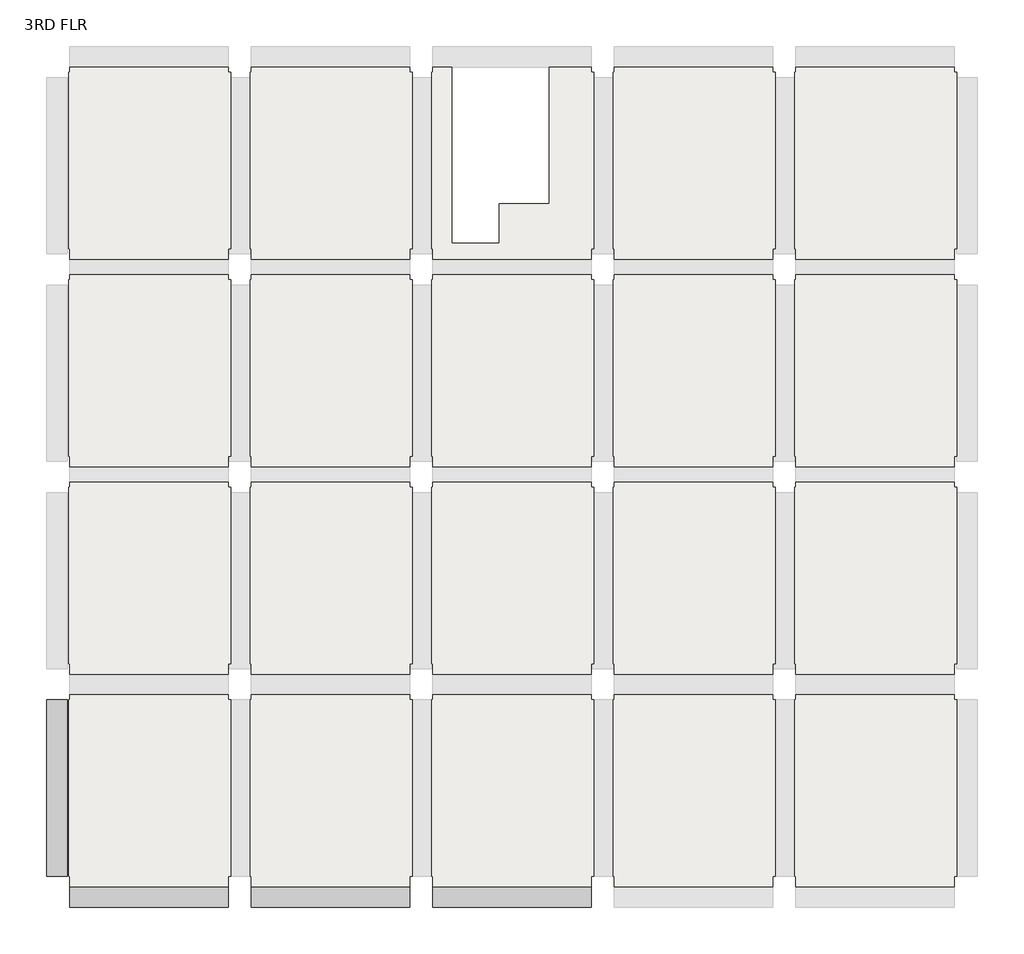
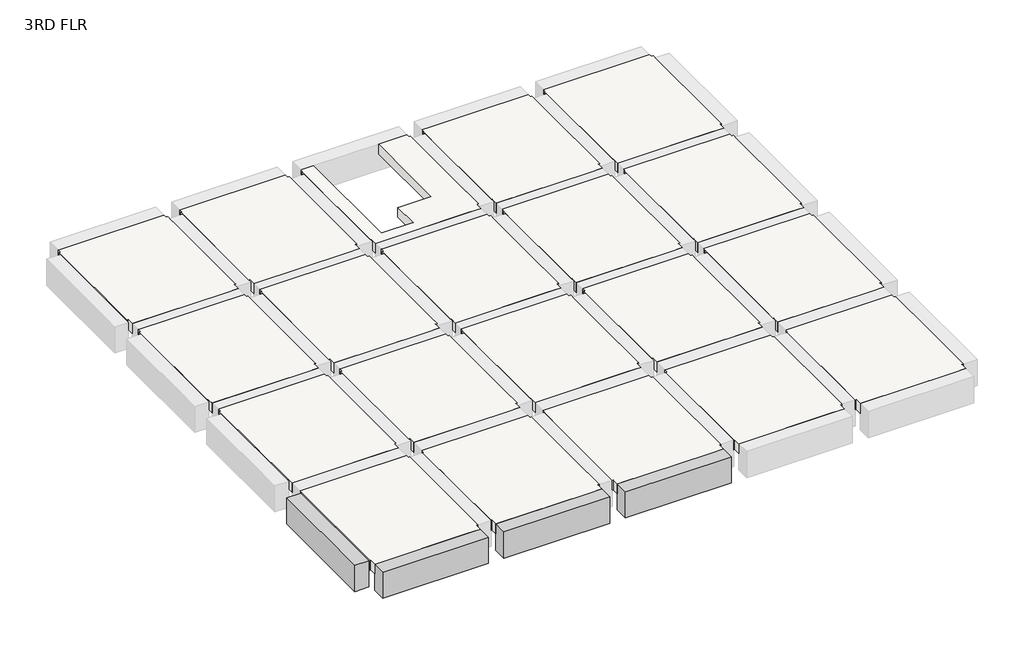
# One storey, part 1 of 2: 20 slabs, 4 beams.
"""IFC4 building model written with IfcOpenShell, lengths in millimetres."""

from ifc_helpers import new_model, si_unit, frame, origin, place, context, project, spatial, polyline, outline, extrude, faceted_brep, element, save

model = new_model("IFC4")

# Units and contexts
model_context = context("Model", 3, world=origin())
ifc_project = project(units=[si_unit("LENGTHUNIT", "METRE", prefix="MILLI")], contexts=[model_context])

# Site, building, storey
site = spatial("IfcSite", under=ifc_project)
building = spatial("IfcBuilding", under=site)
storey = spatial("IfcBuildingStorey", under=building, Name="3RD FLR", Elevation=9144.0)

# Beams
placement = place(None, origin())
element("IfcBeam", 1, ObjectType="M_Concrete-Rectangular Beam : 400 x 800mm", at=placement, inside=storey, context=model_context, shape_type="Brep", body=[
    faceted_brep([(-2144.8884094, 3503.1212443, 9144.0), (-2144.8884094, 3103.1212443, 9144.0), (905.1115906, 3103.1212443, 9144.0), (905.1115906, 3503.1212443, 9144.0), (-2144.8884094, 3503.1212443, 8344.0), (-2144.8884094, 3503.1212443, 8844.0), (905.1115906, 3503.1212443, 8844.0), (905.1115906, 3503.1212443, 8344.0), (-2144.8884094, 3103.1212443, 8344.0), (905.1115906, 3103.1212443, 8344.0)], [[[0, 1, 2, 3]], [[4, 5, 0, 3, 6, 7]], [[8, 4, 7, 9]], [[1, 8, 9, 2]], [[1, 0, 5, 4, 8]], [[3, 2, 9, 7, 6]]]),
])
element("IfcBeam", 2, ObjectType="M_Concrete-Rectangular Beam : 400 x 800mm", at=placement, inside=storey, context=model_context, shape_type="Brep", body=[
    faceted_brep([(-5644.8884094, 3503.1212443, 9144.0), (-5644.8884094, 3103.1212443, 9144.0), (-2594.8884094, 3103.1212443, 9144.0), (-2594.8884094, 3503.1212443, 9144.0), (-5644.8884094, 3503.1212443, 8344.0), (-5644.8884094, 3503.1212443, 8844.0), (-2594.8884094, 3503.1212443, 8844.0), (-2594.8884094, 3503.1212443, 8344.0), (-5644.8884094, 3103.1212443, 8344.0), (-2594.8884094, 3103.1212443, 8344.0)], [[[0, 1, 2, 3]], [[4, 5, 0, 3, 6, 7]], [[8, 4, 7, 9]], [[1, 8, 9, 2]], [[1, 0, 5, 4, 8]], [[3, 2, 9, 7, 6]]]),
])
element("IfcBeam", 3, ObjectType="M_Concrete-Rectangular Beam : 400 x 800mm", at=placement, inside=storey, context=model_context, shape_type="Brep", body=[
    faceted_brep([(-9144.8884094, 3503.1212443, 9144.0), (-9144.8884094, 3103.1212443, 9144.0), (-6094.8884094, 3103.1212443, 9144.0), (-6094.8884094, 3503.1212443, 9144.0), (-9144.8884094, 3503.1212443, 8344.0), (-9144.8884094, 3503.1212443, 8844.0), (-6094.8884094, 3503.1212443, 8844.0), (-6094.8884094, 3503.1212443, 8344.0), (-9144.8884094, 3103.1212443, 8344.0), (-6094.8884094, 3103.1212443, 8344.0)], [[[0, 1, 2, 3]], [[4, 5, 0, 3, 6, 7]], [[8, 4, 7, 9]], [[1, 8, 9, 2]], [[1, 0, 5, 4, 8]], [[3, 2, 9, 7, 6]]]),
])
element("IfcBeam", 4, ObjectType="M_Concrete-Rectangular Beam : 400 x 800mm", at=placement, inside=storey, context=model_context, shape_type="SweptSolid", body=[
    extrude(outline(polyline([(-9594.8884094, 7103.1212443), (-9194.8884094, 7103.1212443), (-9194.8884094, 3703.1212443), (-9594.8884094, 3703.1212443), (-9594.8884094, 7103.1212443)])), frame((0.0, 0.0, 8344.0), z_axis=(0.0, 0.0, 1.0), x_axis=(1.0, 0.0, 0.0)), (0.0, 0.0, 1.0), 800.0),
])

# Slabs
element("IfcSlab", 5, ObjectType="Generic 300mm", at=placement, inside=storey, context=model_context, shape_type="SweptSolid", body=[
    extrude(outline(polyline([(7955.1115906, 7103.1212443), (7955.1115906, 3703.1212443), (7905.1115906, 3703.1212443), (7905.1115906, 3503.1212443), (7530.1115906, 3503.1212443), (4855.1115906, 3503.1212443), (4855.1115906, 3703.1212443), (4830.1115906, 3703.1212443), (4830.1115906, 7103.1212443), (4855.1115906, 7103.1212443), (4855.1115906, 7203.1212443), (7905.1115906, 7203.1212443), (7905.1115906, 7103.1212443), (7955.1115906, 7103.1212443)])), frame((0.0, 0.0, 8844.0), z_axis=(0.0, 0.0, 1.0), x_axis=(1.0, 0.0, 0.0)), (0.0, 0.0, 1.0), 300.0),
])
element("IfcSlab", 6, ObjectType="Generic 300mm", at=placement, inside=storey, context=model_context, shape_type="Brep", body=[
    faceted_brep([(7955.1115906, 11203.1212443, 8844.0), (7955.1115906, 11103.1212443, 8844.0), (7955.1115906, 7803.1212443, 8844.0), (7905.1115906, 7803.1212443, 8844.0), (7905.1115906, 7603.1212443, 8844.0), (7530.1115906, 7603.1212443, 8844.0), (4855.1115906, 7603.1212443, 8844.0), (4855.1115906, 7803.1212443, 8844.0), (4830.1115906, 7803.1212443, 8844.0), (4830.1115906, 11103.1212443, 8844.0), (4830.1115906, 11203.1212443, 8844.0), (4855.1115906, 11203.1212443, 8844.0), (4855.1115906, 11303.1212443, 8844.0), (7905.1115906, 11303.1212443, 8844.0), (7905.1115906, 11203.1212443, 8844.0), (7955.1115906, 11203.1212443, 9144.0), (7905.1115906, 11203.1212443, 9144.0), (7905.1115906, 11303.1212443, 9144.0), (4855.1115906, 11303.1212443, 9144.0), (4855.1115906, 11203.1212443, 9144.0), (4830.1115906, 11203.1212443, 9144.0), (4830.1115906, 11103.1212443, 9144.0), (4830.1115906, 7803.1212443, 9144.0), (4855.1115906, 7803.1212443, 9144.0), (4855.1115906, 7703.1212443, 9144.0), (4855.1115906, 7603.1212443, 9144.0), (7530.1115906, 7603.1212443, 9144.0), (7905.1115906, 7603.1212443, 9144.0), (7905.1115906, 7703.1212443, 9144.0), (7905.1115906, 7803.1212443, 9144.0), (7955.1115906, 7803.1212443, 9144.0), (7955.1115906, 11103.1212443, 9144.0)], [[[0, 1, 2, 3, 4, 5, 6, 7, 8, 9, 10, 11, 12, 13, 14]], [[15, 16, 17, 18, 19, 20, 21, 22, 23, 24, 25, 26, 27, 28, 29, 30, 31]], [[2, 1, 0, 15, 31, 30]], [[3, 2, 30, 29]], [[4, 3, 29, 28, 27]], [[5, 4, 27, 26]], [[6, 5, 26, 25]], [[7, 6, 25, 24, 23]], [[8, 7, 23, 22]], [[10, 9, 8, 22, 21, 20]], [[11, 10, 20, 19]], [[12, 11, 19, 18]], [[13, 12, 18, 17]], [[14, 13, 17, 16]], [[0, 14, 16, 15]]]),
])
element("IfcSlab", 7, ObjectType="Generic 300mm", at=placement, inside=storey, context=model_context, shape_type="Brep", body=[
    faceted_brep([(4455.1115906, 11203.1212443, 8844.0), (4455.1115906, 11103.1212443, 8844.0), (4455.1115906, 7803.1212443, 8844.0), (4430.1115906, 7803.1212443, 8844.0), (4405.1115906, 7803.1212443, 8844.0), (4405.1115906, 7603.1212443, 8844.0), (4030.1115906, 7603.1212443, 8844.0), (1355.1115906, 7603.1212443, 8844.0), (1355.1115906, 7803.1212443, 8844.0), (1330.1115906, 7803.1212443, 8844.0), (1330.1115906, 11103.1212443, 8844.0), (1330.1115906, 11203.1212443, 8844.0), (1355.1115906, 11203.1212443, 8844.0), (1355.1115906, 11303.1212443, 8844.0), (4405.1115906, 11303.1212443, 8844.0), (4405.1115906, 11203.1212443, 8844.0), (4455.1115906, 11203.1212443, 9144.0), (4405.1115906, 11203.1212443, 9144.0), (4405.1115906, 11303.1212443, 9144.0), (1355.1115906, 11303.1212443, 9144.0), (1355.1115906, 11203.1212443, 9144.0), (1330.1115906, 11203.1212443, 9144.0), (1330.1115906, 11103.1212443, 9144.0), (1330.1115906, 7803.1212443, 9144.0), (1355.1115906, 7803.1212443, 9144.0), (1355.1115906, 7703.1212443, 9144.0), (1355.1115906, 7603.1212443, 9144.0), (4030.1115906, 7603.1212443, 9144.0), (4405.1115906, 7603.1212443, 9144.0), (4405.1115906, 7703.1212443, 9144.0), (4405.1115906, 7803.1212443, 9144.0), (4430.1115906, 7803.1212443, 9144.0), (4455.1115906, 7803.1212443, 9144.0), (4455.1115906, 11103.1212443, 9144.0)], [[[0, 1, 2, 3, 4, 5, 6, 7, 8, 9, 10, 11, 12, 13, 14, 15]], [[16, 17, 18, 19, 20, 21, 22, 23, 24, 25, 26, 27, 28, 29, 30, 31, 32, 33]], [[2, 1, 0, 16, 33, 32]], [[4, 3, 2, 32, 31, 30]], [[5, 4, 30, 29, 28]], [[6, 5, 28, 27]], [[7, 6, 27, 26]], [[8, 7, 26, 25, 24]], [[9, 8, 24, 23]], [[11, 10, 9, 23, 22, 21]], [[12, 11, 21, 20]], [[13, 12, 20, 19]], [[14, 13, 19, 18]], [[15, 14, 18, 17]], [[0, 15, 17, 16]]]),
])
element("IfcSlab", 8, ObjectType="Generic 300mm", at=placement, inside=storey, context=model_context, shape_type="Brep", body=[
    faceted_brep([(955.1115906, 11203.1212443, 8844.0), (955.1115906, 11103.1212443, 8844.0), (955.1115906, 7803.1212443, 8844.0), (930.1115906, 7803.1212443, 8844.0), (905.1115906, 7803.1212443, 8844.0), (905.1115906, 7603.1212443, 8844.0), (530.1115906, 7603.1212443, 8844.0), (-2144.8884094, 7603.1212443, 8844.0), (-2144.8884094, 7803.1212443, 8844.0), (-2169.8884094, 7803.1212443, 8844.0), (-2169.8884094, 11103.1212443, 8844.0), (-2169.8884094, 11203.1212443, 8844.0), (-2144.8884094, 11203.1212443, 8844.0), (-2144.8884094, 11303.1212443, 8844.0), (905.1115906, 11303.1212443, 8844.0), (905.1115906, 11203.1212443, 8844.0), (955.1115906, 11203.1212443, 9144.0), (905.1115906, 11203.1212443, 9144.0), (905.1115906, 11303.1212443, 9144.0), (-2144.8884094, 11303.1212443, 9144.0), (-2144.8884094, 11203.1212443, 9144.0), (-2169.8884094, 11203.1212443, 9144.0), (-2169.8884094, 11103.1212443, 9144.0), (-2169.8884094, 7803.1212443, 9144.0), (-2144.8884094, 7803.1212443, 9144.0), (-2144.8884094, 7703.1212443, 9144.0), (-2144.8884094, 7603.1212443, 9144.0), (530.1115906, 7603.1212443, 9144.0), (905.1115906, 7603.1212443, 9144.0), (905.1115906, 7703.1212443, 9144.0), (905.1115906, 7803.1212443, 9144.0), (930.1115906, 7803.1212443, 9144.0), (955.1115906, 7803.1212443, 9144.0), (955.1115906, 11103.1212443, 9144.0)], [[[0, 1, 2, 3, 4, 5, 6, 7, 8, 9, 10, 11, 12, 13, 14, 15]], [[16, 17, 18, 19, 20, 21, 22, 23, 24, 25, 26, 27, 28, 29, 30, 31, 32, 33]], [[2, 1, 0, 16, 33, 32]], [[4, 3, 2, 32, 31, 30]], [[5, 4, 30, 29, 28]], [[6, 5, 28, 27]], [[7, 6, 27, 26]], [[8, 7, 26, 25, 24]], [[9, 8, 24, 23]], [[11, 10, 9, 23, 22, 21]], [[12, 11, 21, 20]], [[13, 12, 20, 19]], [[14, 13, 19, 18]], [[15, 14, 18, 17]], [[0, 15, 17, 16]]]),
])
element("IfcSlab", 9, ObjectType="Generic 300mm", at=placement, inside=storey, context=model_context, shape_type="Brep", body=[
    faceted_brep([(-2544.8884094, 11203.1212443, 8844.0), (-2544.8884094, 11103.1212443, 8844.0), (-2544.8884094, 7803.1212443, 8844.0), (-2569.8884094, 7803.1212443, 8844.0), (-2594.8884094, 7803.1212443, 8844.0), (-2594.8884094, 7603.1212443, 8844.0), (-2969.8884094, 7603.1212443, 8844.0), (-5644.8884094, 7603.1212443, 8844.0), (-5644.8884094, 7803.1212443, 8844.0), (-5669.8884094, 7803.1212443, 8844.0), (-5669.8884094, 11103.1212443, 8844.0), (-5669.8884094, 11203.1212443, 8844.0), (-5644.8884094, 11203.1212443, 8844.0), (-5644.8884094, 11303.1212443, 8844.0), (-2594.8884094, 11303.1212443, 8844.0), (-2594.8884094, 11203.1212443, 8844.0), (-2544.8884094, 11203.1212443, 9144.0), (-2594.8884094, 11203.1212443, 9144.0), (-2594.8884094, 11303.1212443, 9144.0), (-5644.8884094, 11303.1212443, 9144.0), (-5644.8884094, 11203.1212443, 9144.0), (-5669.8884094, 11203.1212443, 9144.0), (-5669.8884094, 11103.1212443, 9144.0), (-5669.8884094, 7803.1212443, 9144.0), (-5644.8884094, 7803.1212443, 9144.0), (-5644.8884094, 7703.1212443, 9144.0), (-5644.8884094, 7603.1212443, 9144.0), (-2969.8884094, 7603.1212443, 9144.0), (-2594.8884094, 7603.1212443, 9144.0), (-2594.8884094, 7703.1212443, 9144.0), (-2594.8884094, 7803.1212443, 9144.0), (-2569.8884094, 7803.1212443, 9144.0), (-2544.8884094, 7803.1212443, 9144.0), (-2544.8884094, 11103.1212443, 9144.0)], [[[0, 1, 2, 3, 4, 5, 6, 7, 8, 9, 10, 11, 12, 13, 14, 15]], [[16, 17, 18, 19, 20, 21, 22, 23, 24, 25, 26, 27, 28, 29, 30, 31, 32, 33]], [[2, 1, 0, 16, 33, 32]], [[4, 3, 2, 32, 31, 30]], [[5, 4, 30, 29, 28]], [[6, 5, 28, 27]], [[7, 6, 27, 26]], [[8, 7, 26, 25, 24]], [[9, 8, 24, 23]], [[11, 10, 9, 23, 22, 21]], [[12, 11, 21, 20]], [[13, 12, 20, 19]], [[14, 13, 19, 18]], [[15, 14, 18, 17]], [[0, 15, 17, 16]]]),
])
element("IfcSlab", 10, ObjectType="Generic 300mm", at=placement, inside=storey, context=model_context, shape_type="Brep", body=[
    faceted_brep([(-6044.8884094, 11203.1212443, 8844.0), (-6044.8884094, 11103.1212443, 8844.0), (-6044.8884094, 7803.1212443, 8844.0), (-6069.8884094, 7803.1212443, 8844.0), (-6094.8884094, 7803.1212443, 8844.0), (-6094.8884094, 7603.1212443, 8844.0), (-6469.8884094, 7603.1212443, 8844.0), (-9144.8884094, 7603.1212443, 8844.0), (-9144.8884094, 7803.1212443, 8844.0), (-9169.8884094, 7803.1212443, 8844.0), (-9169.8884094, 11103.1212443, 8844.0), (-9169.8884094, 11203.1212443, 8844.0), (-9144.8884094, 11203.1212443, 8844.0), (-9144.8884094, 11303.1212443, 8844.0), (-6094.8884094, 11303.1212443, 8844.0), (-6094.8884094, 11203.1212443, 8844.0), (-6044.8884094, 11203.1212443, 9144.0), (-6094.8884094, 11203.1212443, 9144.0), (-6094.8884094, 11303.1212443, 9144.0), (-9144.8884094, 11303.1212443, 9144.0), (-9144.8884094, 11203.1212443, 9144.0), (-9169.8884094, 11203.1212443, 9144.0), (-9169.8884094, 11103.1212443, 9144.0), (-9169.8884094, 7803.1212443, 9144.0), (-9144.8884094, 7803.1212443, 9144.0), (-9144.8884094, 7703.1212443, 9144.0), (-9144.8884094, 7603.1212443, 9144.0), (-6469.8884094, 7603.1212443, 9144.0), (-6094.8884094, 7603.1212443, 9144.0), (-6094.8884094, 7703.1212443, 9144.0), (-6094.8884094, 7803.1212443, 9144.0), (-6069.8884094, 7803.1212443, 9144.0), (-6044.8884094, 7803.1212443, 9144.0), (-6044.8884094, 11103.1212443, 9144.0)], [[[0, 1, 2, 3, 4, 5, 6, 7, 8, 9, 10, 11, 12, 13, 14, 15]], [[16, 17, 18, 19, 20, 21, 22, 23, 24, 25, 26, 27, 28, 29, 30, 31, 32, 33]], [[2, 1, 0, 16, 33, 32]], [[4, 3, 2, 32, 31, 30]], [[5, 4, 30, 29, 28]], [[6, 5, 28, 27]], [[7, 6, 27, 26]], [[8, 7, 26, 25, 24]], [[9, 8, 24, 23]], [[11, 10, 9, 23, 22, 21]], [[12, 11, 21, 20]], [[13, 12, 20, 19]], [[14, 13, 19, 18]], [[15, 14, 18, 17]], [[0, 15, 17, 16]]]),
])
element("IfcSlab", 11, ObjectType="Generic 300mm", at=placement, inside=storey, context=model_context, shape_type="Brep", body=[
    faceted_brep([(-6044.8884094, 7103.1212443, 8844.0), (-6044.8884094, 3703.1212443, 8844.0), (-6069.8884094, 3703.1212443, 8844.0), (-6094.8884094, 3703.1212443, 8844.0), (-6094.8884094, 3503.1212443, 8844.0), (-6469.8884094, 3503.1212443, 8844.0), (-9144.8884094, 3503.1212443, 8844.0), (-9144.8884094, 3703.1212443, 8844.0), (-9169.8884094, 3703.1212443, 8844.0), (-9169.8884094, 7103.1212443, 8844.0), (-9144.8884094, 7103.1212443, 8844.0), (-9144.8884094, 7203.1212443, 8844.0), (-6094.8884094, 7203.1212443, 8844.0), (-6094.8884094, 7103.1212443, 8844.0), (-6069.8884094, 7103.1212443, 8844.0), (-6044.8884094, 7103.1212443, 9144.0), (-6094.8884094, 7103.1212443, 9144.0), (-6094.8884094, 7203.1212443, 9144.0), (-9144.8884094, 7203.1212443, 9144.0), (-9144.8884094, 7103.1212443, 9144.0), (-9169.8884094, 7103.1212443, 9144.0), (-9169.8884094, 3703.1212443, 9144.0), (-9144.8884094, 3703.1212443, 9144.0), (-9144.8884094, 3503.1212443, 9144.0), (-6469.8884094, 3503.1212443, 9144.0), (-6094.8884094, 3503.1212443, 9144.0), (-6094.8884094, 3703.1212443, 9144.0), (-6044.8884094, 3703.1212443, 9144.0)], [[[0, 1, 2, 3, 4, 5, 6, 7, 8, 9, 10, 11, 12, 13, 14]], [[15, 16, 17, 18, 19, 20, 21, 22, 23, 24, 25, 26, 27]], [[1, 0, 15, 27]], [[3, 2, 1, 27, 26]], [[4, 3, 26, 25]], [[5, 4, 25, 24]], [[6, 5, 24, 23]], [[7, 6, 23, 22]], [[8, 7, 22, 21]], [[9, 8, 21, 20]], [[10, 9, 20, 19]], [[11, 10, 19, 18]], [[12, 11, 18, 17]], [[13, 12, 17, 16]], [[0, 14, 13, 16, 15]]]),
])
element("IfcSlab", 12, ObjectType="Generic 300mm", at=placement, inside=storey, context=model_context, shape_type="Brep", body=[
    faceted_brep([(-2544.8884094, 7103.1212443, 8844.0), (-2544.8884094, 3703.1212443, 8844.0), (-2569.8884094, 3703.1212443, 8844.0), (-2594.8884094, 3703.1212443, 8844.0), (-2594.8884094, 3503.1212443, 8844.0), (-2969.8884094, 3503.1212443, 8844.0), (-5644.8884094, 3503.1212443, 8844.0), (-5644.8884094, 3703.1212443, 8844.0), (-5669.8884094, 3703.1212443, 8844.0), (-5669.8884094, 7103.1212443, 8844.0), (-5644.8884094, 7103.1212443, 8844.0), (-5644.8884094, 7203.1212443, 8844.0), (-2594.8884094, 7203.1212443, 8844.0), (-2594.8884094, 7103.1212443, 8844.0), (-2569.8884094, 7103.1212443, 8844.0), (-2544.8884094, 7103.1212443, 9144.0), (-2594.8884094, 7103.1212443, 9144.0), (-2594.8884094, 7203.1212443, 9144.0), (-5644.8884094, 7203.1212443, 9144.0), (-5644.8884094, 7103.1212443, 9144.0), (-5669.8884094, 7103.1212443, 9144.0), (-5669.8884094, 3703.1212443, 9144.0), (-5644.8884094, 3703.1212443, 9144.0), (-5644.8884094, 3503.1212443, 9144.0), (-2969.8884094, 3503.1212443, 9144.0), (-2594.8884094, 3503.1212443, 9144.0), (-2594.8884094, 3703.1212443, 9144.0), (-2544.8884094, 3703.1212443, 9144.0)], [[[0, 1, 2, 3, 4, 5, 6, 7, 8, 9, 10, 11, 12, 13, 14]], [[15, 16, 17, 18, 19, 20, 21, 22, 23, 24, 25, 26, 27]], [[1, 0, 15, 27]], [[3, 2, 1, 27, 26]], [[4, 3, 26, 25]], [[5, 4, 25, 24]], [[6, 5, 24, 23]], [[7, 6, 23, 22]], [[8, 7, 22, 21]], [[9, 8, 21, 20]], [[10, 9, 20, 19]], [[11, 10, 19, 18]], [[12, 11, 18, 17]], [[13, 12, 17, 16]], [[0, 14, 13, 16, 15]]]),
])
element("IfcSlab", 13, ObjectType="Generic 300mm", at=placement, inside=storey, context=model_context, shape_type="Brep", body=[
    faceted_brep([(955.1115906, 7103.1212443, 8844.0), (955.1115906, 3703.1212443, 8844.0), (930.1115906, 3703.1212443, 8844.0), (905.1115906, 3703.1212443, 8844.0), (905.1115906, 3503.1212443, 8844.0), (530.1115906, 3503.1212443, 8844.0), (-2144.8884094, 3503.1212443, 8844.0), (-2144.8884094, 3703.1212443, 8844.0), (-2169.8884094, 3703.1212443, 8844.0), (-2169.8884094, 7103.1212443, 8844.0), (-2144.8884094, 7103.1212443, 8844.0), (-2144.8884094, 7203.1212443, 8844.0), (905.1115906, 7203.1212443, 8844.0), (905.1115906, 7103.1212443, 8844.0), (930.1115906, 7103.1212443, 8844.0), (955.1115906, 7103.1212443, 9144.0), (905.1115906, 7103.1212443, 9144.0), (905.1115906, 7203.1212443, 9144.0), (-2144.8884094, 7203.1212443, 9144.0), (-2144.8884094, 7103.1212443, 9144.0), (-2169.8884094, 7103.1212443, 9144.0), (-2169.8884094, 3703.1212443, 9144.0), (-2144.8884094, 3703.1212443, 9144.0), (-2144.8884094, 3503.1212443, 9144.0), (530.1115906, 3503.1212443, 9144.0), (905.1115906, 3503.1212443, 9144.0), (905.1115906, 3703.1212443, 9144.0), (955.1115906, 3703.1212443, 9144.0)], [[[0, 1, 2, 3, 4, 5, 6, 7, 8, 9, 10, 11, 12, 13, 14]], [[15, 16, 17, 18, 19, 20, 21, 22, 23, 24, 25, 26, 27]], [[1, 0, 15, 27]], [[3, 2, 1, 27, 26]], [[4, 3, 26, 25]], [[5, 4, 25, 24]], [[6, 5, 24, 23]], [[7, 6, 23, 22]], [[8, 7, 22, 21]], [[9, 8, 21, 20]], [[10, 9, 20, 19]], [[11, 10, 19, 18]], [[12, 11, 18, 17]], [[13, 12, 17, 16]], [[0, 14, 13, 16, 15]]]),
])
element("IfcSlab", 14, ObjectType="Generic 300mm", at=placement, inside=storey, context=model_context, shape_type="Brep", body=[
    faceted_brep([(4455.1115906, 7103.1212443, 8844.0), (4455.1115906, 3703.1212443, 8844.0), (4430.1115906, 3703.1212443, 8844.0), (4405.1115906, 3703.1212443, 8844.0), (4405.1115906, 3503.1212443, 8844.0), (4030.1115906, 3503.1212443, 8844.0), (1355.1115906, 3503.1212443, 8844.0), (1355.1115906, 3703.1212443, 8844.0), (1330.1115906, 3703.1212443, 8844.0), (1330.1115906, 7103.1212443, 8844.0), (1355.1115906, 7103.1212443, 8844.0), (1355.1115906, 7203.1212443, 8844.0), (4405.1115906, 7203.1212443, 8844.0), (4405.1115906, 7103.1212443, 8844.0), (4430.1115906, 7103.1212443, 8844.0), (4455.1115906, 7103.1212443, 9144.0), (4405.1115906, 7103.1212443, 9144.0), (4405.1115906, 7203.1212443, 9144.0), (1355.1115906, 7203.1212443, 9144.0), (1355.1115906, 7103.1212443, 9144.0), (1330.1115906, 7103.1212443, 9144.0), (1330.1115906, 3703.1212443, 9144.0), (1355.1115906, 3703.1212443, 9144.0), (1355.1115906, 3503.1212443, 9144.0), (4030.1115906, 3503.1212443, 9144.0), (4405.1115906, 3503.1212443, 9144.0), (4405.1115906, 3703.1212443, 9144.0), (4455.1115906, 3703.1212443, 9144.0)], [[[0, 1, 2, 3, 4, 5, 6, 7, 8, 9, 10, 11, 12, 13, 14]], [[15, 16, 17, 18, 19, 20, 21, 22, 23, 24, 25, 26, 27]], [[1, 0, 15, 27]], [[3, 2, 1, 27, 26]], [[4, 3, 26, 25]], [[5, 4, 25, 24]], [[6, 5, 24, 23]], [[7, 6, 23, 22]], [[8, 7, 22, 21]], [[9, 8, 21, 20]], [[10, 9, 20, 19]], [[11, 10, 19, 18]], [[12, 11, 18, 17]], [[13, 12, 17, 16]], [[0, 14, 13, 16, 15]]]),
])
element("IfcSlab", 15, ObjectType="Generic 300mm", at=placement, inside=storey, context=model_context, shape_type="Brep", body=[
    faceted_brep([(7955.1115906, 15203.1212443, 8844.0), (7955.1115906, 15103.1212443, 8844.0), (7955.1115906, 11803.1212443, 8844.0), (7905.1115906, 11803.1212443, 8844.0), (7905.1115906, 11603.1212443, 8844.0), (7530.1115906, 11603.1212443, 8844.0), (4855.1115906, 11603.1212443, 8844.0), (4855.1115906, 11803.1212443, 8844.0), (4830.1115906, 11803.1212443, 8844.0), (4830.1115906, 15103.1212443, 8844.0), (4830.1115906, 15203.1212443, 8844.0), (4855.1115906, 15203.1212443, 8844.0), (4855.1115906, 15303.1212443, 8844.0), (7905.1115906, 15303.1212443, 8844.0), (7905.1115906, 15203.1212443, 8844.0), (7955.1115906, 15203.1212443, 9144.0), (7905.1115906, 15203.1212443, 9144.0), (7905.1115906, 15303.1212443, 9144.0), (4855.1115906, 15303.1212443, 9144.0), (4855.1115906, 15203.1212443, 9144.0), (4830.1115906, 15203.1212443, 9144.0), (4830.1115906, 15103.1212443, 9144.0), (4830.1115906, 11803.1212443, 9144.0), (4855.1115906, 11803.1212443, 9144.0), (4855.1115906, 11703.1212443, 9144.0), (4855.1115906, 11603.1212443, 9144.0), (7530.1115906, 11603.1212443, 9144.0), (7905.1115906, 11603.1212443, 9144.0), (7905.1115906, 11703.1212443, 9144.0), (7905.1115906, 11803.1212443, 9144.0), (7955.1115906, 11803.1212443, 9144.0), (7955.1115906, 15103.1212443, 9144.0)], [[[0, 1, 2, 3, 4, 5, 6, 7, 8, 9, 10, 11, 12, 13, 14]], [[15, 16, 17, 18, 19, 20, 21, 22, 23, 24, 25, 26, 27, 28, 29, 30, 31]], [[2, 1, 0, 15, 31, 30]], [[3, 2, 30, 29]], [[4, 3, 29, 28, 27]], [[5, 4, 27, 26]], [[6, 5, 26, 25]], [[7, 6, 25, 24, 23]], [[8, 7, 23, 22]], [[10, 9, 8, 22, 21, 20]], [[11, 10, 20, 19]], [[12, 11, 19, 18]], [[13, 12, 18, 17]], [[14, 13, 17, 16]], [[0, 14, 16, 15]]]),
])
element("IfcSlab", 16, ObjectType="Generic 300mm", at=placement, inside=storey, context=model_context, shape_type="Brep", body=[
    faceted_brep([(7955.1115906, 19203.1212443, 8844.0), (7955.1115906, 19103.1212443, 8844.0), (7955.1115906, 15803.1212443, 8844.0), (7905.1115906, 15803.1212443, 8844.0), (7905.1115906, 15603.1212443, 8844.0), (7530.1115906, 15603.1212443, 8844.0), (4855.1115906, 15603.1212443, 8844.0), (4855.1115906, 15803.1212443, 8844.0), (4830.1115906, 15803.1212443, 8844.0), (4830.1115906, 19103.1212443, 8844.0), (4830.1115906, 19203.1212443, 8844.0), (4855.1115906, 19203.1212443, 8844.0), (4855.1115906, 19303.1212443, 8844.0), (7905.1115906, 19303.1212443, 8844.0), (7905.1115906, 19203.1212443, 8844.0), (7955.1115906, 19203.1212443, 9144.0), (7905.1115906, 19203.1212443, 9144.0), (7905.1115906, 19303.1212443, 9144.0), (4855.1115906, 19303.1212443, 9144.0), (4855.1115906, 19203.1212443, 9144.0), (4830.1115906, 19203.1212443, 9144.0), (4830.1115906, 19103.1212443, 9144.0), (4830.1115906, 15803.1212443, 9144.0), (4855.1115906, 15803.1212443, 9144.0), (4855.1115906, 15703.1212443, 9144.0), (4855.1115906, 15603.1212443, 9144.0), (7530.1115906, 15603.1212443, 9144.0), (7905.1115906, 15603.1212443, 9144.0), (7905.1115906, 15703.1212443, 9144.0), (7905.1115906, 15803.1212443, 9144.0), (7955.1115906, 15803.1212443, 9144.0), (7955.1115906, 19103.1212443, 9144.0)], [[[0, 1, 2, 3, 4, 5, 6, 7, 8, 9, 10, 11, 12, 13, 14]], [[15, 16, 17, 18, 19, 20, 21, 22, 23, 24, 25, 26, 27, 28, 29, 30, 31]], [[2, 1, 0, 15, 31, 30]], [[3, 2, 30, 29]], [[4, 3, 29, 28, 27]], [[5, 4, 27, 26]], [[6, 5, 26, 25]], [[7, 6, 25, 24, 23]], [[8, 7, 23, 22]], [[10, 9, 8, 22, 21, 20]], [[11, 10, 20, 19]], [[12, 11, 19, 18]], [[13, 12, 18, 17]], [[14, 13, 17, 16]], [[0, 14, 16, 15]]]),
])
element("IfcSlab", 17, ObjectType="Generic 300mm", at=placement, inside=storey, context=model_context, shape_type="Brep", body=[
    faceted_brep([(4455.1115906, 19203.1212443, 8844.0), (4455.1115906, 19103.1212443, 8844.0), (4455.1115906, 15803.1212443, 8844.0), (4430.1115906, 15803.1212443, 8844.0), (4405.1115906, 15803.1212443, 8844.0), (4405.1115906, 15603.1212443, 8844.0), (4030.1115906, 15603.1212443, 8844.0), (1355.1115906, 15603.1212443, 8844.0), (1355.1115906, 15803.1212443, 8844.0), (1330.1115906, 15803.1212443, 8844.0), (1330.1115906, 19103.1212443, 8844.0), (1330.1115906, 19203.1212443, 8844.0), (1355.1115906, 19203.1212443, 8844.0), (1355.1115906, 19303.1212443, 8844.0), (4405.1115906, 19303.1212443, 8844.0), (4405.1115906, 19203.1212443, 8844.0), (4455.1115906, 19203.1212443, 9144.0), (4405.1115906, 19203.1212443, 9144.0), (4405.1115906, 19303.1212443, 9144.0), (1355.1115906, 19303.1212443, 9144.0), (1355.1115906, 19203.1212443, 9144.0), (1330.1115906, 19203.1212443, 9144.0), (1330.1115906, 19103.1212443, 9144.0), (1330.1115906, 15803.1212443, 9144.0), (1355.1115906, 15803.1212443, 9144.0), (1355.1115906, 15703.1212443, 9144.0), (1355.1115906, 15603.1212443, 9144.0), (4030.1115906, 15603.1212443, 9144.0), (4405.1115906, 15603.1212443, 9144.0), (4405.1115906, 15703.1212443, 9144.0), (4405.1115906, 15803.1212443, 9144.0), (4430.1115906, 15803.1212443, 9144.0), (4455.1115906, 15803.1212443, 9144.0), (4455.1115906, 19103.1212443, 9144.0)], [[[0, 1, 2, 3, 4, 5, 6, 7, 8, 9, 10, 11, 12, 13, 14, 15]], [[16, 17, 18, 19, 20, 21, 22, 23, 24, 25, 26, 27, 28, 29, 30, 31, 32, 33]], [[2, 1, 0, 16, 33, 32]], [[4, 3, 2, 32, 31, 30]], [[5, 4, 30, 29, 28]], [[6, 5, 28, 27]], [[7, 6, 27, 26]], [[8, 7, 26, 25, 24]], [[9, 8, 24, 23]], [[11, 10, 9, 23, 22, 21]], [[12, 11, 21, 20]], [[13, 12, 20, 19]], [[14, 13, 19, 18]], [[15, 14, 18, 17]], [[0, 15, 17, 16]]]),
])
element("IfcSlab", 18, ObjectType="Generic 300mm", at=placement, inside=storey, context=model_context, shape_type="Brep", body=[
    faceted_brep([(4455.1115906, 15203.1212443, 8844.0), (4455.1115906, 15103.1212443, 8844.0), (4455.1115906, 11803.1212443, 8844.0), (4430.1115906, 11803.1212443, 8844.0), (4405.1115906, 11803.1212443, 8844.0), (4405.1115906, 11603.1212443, 8844.0), (4030.1115906, 11603.1212443, 8844.0), (1355.1115906, 11603.1212443, 8844.0), (1355.1115906, 11803.1212443, 8844.0), (1330.1115906, 11803.1212443, 8844.0), (1330.1115906, 15103.1212443, 8844.0), (1330.1115906, 15203.1212443, 8844.0), (1355.1115906, 15203.1212443, 8844.0), (1355.1115906, 15303.1212443, 8844.0), (4405.1115906, 15303.1212443, 8844.0), (4405.1115906, 15203.1212443, 8844.0), (4455.1115906, 15203.1212443, 9144.0), (4405.1115906, 15203.1212443, 9144.0), (4405.1115906, 15303.1212443, 9144.0), (1355.1115906, 15303.1212443, 9144.0), (1355.1115906, 15203.1212443, 9144.0), (1330.1115906, 15203.1212443, 9144.0), (1330.1115906, 15103.1212443, 9144.0), (1330.1115906, 11803.1212443, 9144.0), (1355.1115906, 11803.1212443, 9144.0), (1355.1115906, 11703.1212443, 9144.0), (1355.1115906, 11603.1212443, 9144.0), (4030.1115906, 11603.1212443, 9144.0), (4405.1115906, 11603.1212443, 9144.0), (4405.1115906, 11703.1212443, 9144.0), (4405.1115906, 11803.1212443, 9144.0), (4430.1115906, 11803.1212443, 9144.0), (4455.1115906, 11803.1212443, 9144.0), (4455.1115906, 15103.1212443, 9144.0)], [[[0, 1, 2, 3, 4, 5, 6, 7, 8, 9, 10, 11, 12, 13, 14, 15]], [[16, 17, 18, 19, 20, 21, 22, 23, 24, 25, 26, 27, 28, 29, 30, 31, 32, 33]], [[2, 1, 0, 16, 33, 32]], [[4, 3, 2, 32, 31, 30]], [[5, 4, 30, 29, 28]], [[6, 5, 28, 27]], [[7, 6, 27, 26]], [[8, 7, 26, 25, 24]], [[9, 8, 24, 23]], [[11, 10, 9, 23, 22, 21]], [[12, 11, 21, 20]], [[13, 12, 20, 19]], [[14, 13, 19, 18]], [[15, 14, 18, 17]], [[0, 15, 17, 16]]]),
])
element("IfcSlab", 19, ObjectType="Generic 300mm", at=placement, inside=storey, context=model_context, shape_type="Brep", body=[
    faceted_brep([(955.1115906, 15203.1212443, 8844.0), (955.1115906, 15103.1212443, 8844.0), (955.1115906, 11803.1212443, 8844.0), (930.1115906, 11803.1212443, 8844.0), (905.1115906, 11803.1212443, 8844.0), (905.1115906, 11603.1212443, 8844.0), (530.1115906, 11603.1212443, 8844.0), (-2144.8884094, 11603.1212443, 8844.0), (-2144.8884094, 11803.1212443, 8844.0), (-2169.8884094, 11803.1212443, 8844.0), (-2169.8884094, 15103.1212443, 8844.0), (-2169.8884094, 15203.1212443, 8844.0), (-2144.8884094, 15203.1212443, 8844.0), (-2144.8884094, 15303.1212443, 8844.0), (905.1115906, 15303.1212443, 8844.0), (905.1115906, 15203.1212443, 8844.0), (955.1115906, 15203.1212443, 9144.0), (905.1115906, 15203.1212443, 9144.0), (905.1115906, 15303.1212443, 9144.0), (-2144.8884094, 15303.1212443, 9144.0), (-2144.8884094, 15203.1212443, 9144.0), (-2169.8884094, 15203.1212443, 9144.0), (-2169.8884094, 15103.1212443, 9144.0), (-2169.8884094, 11803.1212443, 9144.0), (-2144.8884094, 11803.1212443, 9144.0), (-2144.8884094, 11703.1212443, 9144.0), (-2144.8884094, 11603.1212443, 9144.0), (530.1115906, 11603.1212443, 9144.0), (905.1115906, 11603.1212443, 9144.0), (905.1115906, 11703.1212443, 9144.0), (905.1115906, 11803.1212443, 9144.0), (930.1115906, 11803.1212443, 9144.0), (955.1115906, 11803.1212443, 9144.0), (955.1115906, 15103.1212443, 9144.0)], [[[0, 1, 2, 3, 4, 5, 6, 7, 8, 9, 10, 11, 12, 13, 14, 15]], [[16, 17, 18, 19, 20, 21, 22, 23, 24, 25, 26, 27, 28, 29, 30, 31, 32, 33]], [[2, 1, 0, 16, 33, 32]], [[4, 3, 2, 32, 31, 30]], [[5, 4, 30, 29, 28]], [[6, 5, 28, 27]], [[7, 6, 27, 26]], [[8, 7, 26, 25, 24]], [[9, 8, 24, 23]], [[11, 10, 9, 23, 22, 21]], [[12, 11, 21, 20]], [[13, 12, 20, 19]], [[14, 13, 19, 18]], [[15, 14, 18, 17]], [[0, 15, 17, 16]]]),
])
element("IfcSlab", 20, ObjectType="Generic 300mm", at=placement, inside=storey, context=model_context, shape_type="Brep", body=[
    faceted_brep([(955.1115906, 19203.1212443, 8844.0), (955.1115906, 19103.1212443, 8844.0), (955.1115906, 15803.1212443, 8844.0), (930.1115906, 15803.1212443, 8844.0), (905.1115906, 15803.1212443, 8844.0), (905.1115906, 15603.1212443, 8844.0), (530.1115906, 15603.1212443, 8844.0), (-2144.8884094, 15603.1212443, 8844.0), (-2144.8884094, 15803.1212443, 8844.0), (-2169.8884094, 15803.1212443, 8844.0), (-2169.8884094, 19103.1212443, 8844.0), (-2169.8884094, 19203.1212443, 8844.0), (-2144.8884094, 19203.1212443, 8844.0), (-2144.8884094, 19303.1212443, 8844.0), (-1784.8884094, 19303.1212443, 8844.0), (-1784.8884094, 15908.7212443, 8844.0), (-870.4884094, 15908.7212443, 8844.0), (-870.4884094, 16670.7212443, 8844.0), (-819.6884094, 16670.7212443, 8844.0), (94.7115906, 16670.7212443, 8844.0), (94.7115906, 19303.1212443, 8844.0), (905.1115906, 19303.1212443, 8844.0), (905.1115906, 19203.1212443, 8844.0), (955.1115906, 15803.1212443, 9144.0), (955.1115906, 19103.1212443, 9144.0), (955.1115906, 19203.1212443, 9144.0), (905.1115906, 19203.1212443, 9144.0), (905.1115906, 19303.1212443, 9144.0), (94.7115906, 19303.1212443, 9144.0), (94.7115906, 16670.7212443, 9144.0), (-819.6884094, 16670.7212443, 9144.0), (-870.4884094, 16670.7212443, 9144.0), (-870.4884094, 15908.7212443, 9144.0), (-1784.8884094, 15908.7212443, 9144.0), (-1784.8884094, 19303.1212443, 9144.0), (-2144.8884094, 19303.1212443, 9144.0), (-2144.8884094, 19203.1212443, 9144.0), (-2169.8884094, 19203.1212443, 9144.0), (-2169.8884094, 19103.1212443, 9144.0), (-2169.8884094, 15803.1212443, 9144.0), (-2144.8884094, 15803.1212443, 9144.0), (-2144.8884094, 15703.1212443, 9144.0), (-2144.8884094, 15603.1212443, 9144.0), (530.1115906, 15603.1212443, 9144.0), (905.1115906, 15603.1212443, 9144.0), (905.1115906, 15703.1212443, 9144.0), (905.1115906, 15803.1212443, 9144.0), (930.1115906, 15803.1212443, 9144.0)], [[[0, 1, 2, 3, 4, 5, 6, 7, 8, 9, 10, 11, 12, 13, 14, 15, 16, 17, 18, 19, 20, 21, 22]], [[23, 24, 25, 26, 27, 28, 29, 30, 31, 32, 33, 34, 35, 36, 37, 38, 39, 40, 41, 42, 43, 44, 45, 46, 47]], [[2, 1, 0, 25, 24, 23]], [[4, 3, 2, 23, 47, 46]], [[5, 4, 46, 45, 44]], [[6, 5, 44, 43]], [[7, 6, 43, 42]], [[8, 7, 42, 41, 40]], [[9, 8, 40, 39]], [[11, 10, 9, 39, 38, 37]], [[12, 11, 37, 36]], [[13, 12, 36, 35]], [[13, 35, 34, 14]], [[27, 21, 20, 28]], [[22, 21, 27, 26]], [[0, 22, 26, 25]], [[19, 29, 28, 20]], [[33, 15, 14, 34]], [[15, 33, 32, 16]], [[16, 32, 31, 17]], [[17, 31, 30, 18]], [[29, 19, 18, 30]]]),
])
element("IfcSlab", 21, ObjectType="Generic 300mm", at=placement, inside=storey, context=model_context, shape_type="Brep", body=[
    faceted_brep([(-2544.8884094, 19203.1212443, 8844.0), (-2544.8884094, 19103.1212443, 8844.0), (-2544.8884094, 15803.1212443, 8844.0), (-2569.8884094, 15803.1212443, 8844.0), (-2594.8884094, 15803.1212443, 8844.0), (-2594.8884094, 15603.1212443, 8844.0), (-2969.8884094, 15603.1212443, 8844.0), (-5644.8884094, 15603.1212443, 8844.0), (-5644.8884094, 15803.1212443, 8844.0), (-5669.8884094, 15803.1212443, 8844.0), (-5669.8884094, 19103.1212443, 8844.0), (-5669.8884094, 19203.1212443, 8844.0), (-5644.8884094, 19203.1212443, 8844.0), (-5644.8884094, 19303.1212443, 8844.0), (-2594.8884094, 19303.1212443, 8844.0), (-2594.8884094, 19203.1212443, 8844.0), (-2544.8884094, 19203.1212443, 9144.0), (-2594.8884094, 19203.1212443, 9144.0), (-2594.8884094, 19303.1212443, 9144.0), (-5644.8884094, 19303.1212443, 9144.0), (-5644.8884094, 19203.1212443, 9144.0), (-5669.8884094, 19203.1212443, 9144.0), (-5669.8884094, 19103.1212443, 9144.0), (-5669.8884094, 15803.1212443, 9144.0), (-5644.8884094, 15803.1212443, 9144.0), (-5644.8884094, 15703.1212443, 9144.0), (-5644.8884094, 15603.1212443, 9144.0), (-2969.8884094, 15603.1212443, 9144.0), (-2594.8884094, 15603.1212443, 9144.0), (-2594.8884094, 15703.1212443, 9144.0), (-2594.8884094, 15803.1212443, 9144.0), (-2569.8884094, 15803.1212443, 9144.0), (-2544.8884094, 15803.1212443, 9144.0), (-2544.8884094, 19103.1212443, 9144.0)], [[[0, 1, 2, 3, 4, 5, 6, 7, 8, 9, 10, 11, 12, 13, 14, 15]], [[16, 17, 18, 19, 20, 21, 22, 23, 24, 25, 26, 27, 28, 29, 30, 31, 32, 33]], [[2, 1, 0, 16, 33, 32]], [[4, 3, 2, 32, 31, 30]], [[5, 4, 30, 29, 28]], [[6, 5, 28, 27]], [[7, 6, 27, 26]], [[8, 7, 26, 25, 24]], [[9, 8, 24, 23]], [[11, 10, 9, 23, 22, 21]], [[12, 11, 21, 20]], [[13, 12, 20, 19]], [[14, 13, 19, 18]], [[15, 14, 18, 17]], [[0, 15, 17, 16]]]),
])
element("IfcSlab", 22, ObjectType="Generic 300mm", at=placement, inside=storey, context=model_context, shape_type="Brep", body=[
    faceted_brep([(-6044.8884094, 19203.1212443, 8844.0), (-6044.8884094, 19103.1212443, 8844.0), (-6044.8884094, 15803.1212443, 8844.0), (-6069.8884094, 15803.1212443, 8844.0), (-6094.8884094, 15803.1212443, 8844.0), (-6094.8884094, 15603.1212443, 8844.0), (-6469.8884094, 15603.1212443, 8844.0), (-9144.8884094, 15603.1212443, 8844.0), (-9144.8884094, 15803.1212443, 8844.0), (-9169.8884094, 15803.1212443, 8844.0), (-9169.8884094, 19103.1212443, 8844.0), (-9169.8884094, 19203.1212443, 8844.0), (-9144.8884094, 19203.1212443, 8844.0), (-9144.8884094, 19303.1212443, 8844.0), (-6094.8884094, 19303.1212443, 8844.0), (-6094.8884094, 19203.1212443, 8844.0), (-6044.8884094, 19203.1212443, 9144.0), (-6094.8884094, 19203.1212443, 9144.0), (-6094.8884094, 19303.1212443, 9144.0), (-9144.8884094, 19303.1212443, 9144.0), (-9144.8884094, 19203.1212443, 9144.0), (-9169.8884094, 19203.1212443, 9144.0), (-9169.8884094, 19103.1212443, 9144.0), (-9169.8884094, 15803.1212443, 9144.0), (-9144.8884094, 15803.1212443, 9144.0), (-9144.8884094, 15703.1212443, 9144.0), (-9144.8884094, 15603.1212443, 9144.0), (-6469.8884094, 15603.1212443, 9144.0), (-6094.8884094, 15603.1212443, 9144.0), (-6094.8884094, 15703.1212443, 9144.0), (-6094.8884094, 15803.1212443, 9144.0), (-6069.8884094, 15803.1212443, 9144.0), (-6044.8884094, 15803.1212443, 9144.0), (-6044.8884094, 19103.1212443, 9144.0)], [[[0, 1, 2, 3, 4, 5, 6, 7, 8, 9, 10, 11, 12, 13, 14, 15]], [[16, 17, 18, 19, 20, 21, 22, 23, 24, 25, 26, 27, 28, 29, 30, 31, 32, 33]], [[2, 1, 0, 16, 33, 32]], [[4, 3, 2, 32, 31, 30]], [[5, 4, 30, 29, 28]], [[6, 5, 28, 27]], [[7, 6, 27, 26]], [[8, 7, 26, 25, 24]], [[9, 8, 24, 23]], [[11, 10, 9, 23, 22, 21]], [[12, 11, 21, 20]], [[13, 12, 20, 19]], [[14, 13, 19, 18]], [[15, 14, 18, 17]], [[0, 15, 17, 16]]]),
])
element("IfcSlab", 23, ObjectType="Generic 300mm", at=placement, inside=storey, context=model_context, shape_type="Brep", body=[
    faceted_brep([(-6044.8884094, 15203.1212443, 8844.0), (-6044.8884094, 15103.1212443, 8844.0), (-6044.8884094, 11803.1212443, 8844.0), (-6069.8884094, 11803.1212443, 8844.0), (-6094.8884094, 11803.1212443, 8844.0), (-6094.8884094, 11603.1212443, 8844.0), (-6469.8884094, 11603.1212443, 8844.0), (-9144.8884094, 11603.1212443, 8844.0), (-9144.8884094, 11803.1212443, 8844.0), (-9169.8884094, 11803.1212443, 8844.0), (-9169.8884094, 15103.1212443, 8844.0), (-9169.8884094, 15203.1212443, 8844.0), (-9144.8884094, 15203.1212443, 8844.0), (-9144.8884094, 15303.1212443, 8844.0), (-6094.8884094, 15303.1212443, 8844.0), (-6094.8884094, 15203.1212443, 8844.0), (-6044.8884094, 15203.1212443, 9144.0), (-6094.8884094, 15203.1212443, 9144.0), (-6094.8884094, 15303.1212443, 9144.0), (-9144.8884094, 15303.1212443, 9144.0), (-9144.8884094, 15203.1212443, 9144.0), (-9169.8884094, 15203.1212443, 9144.0), (-9169.8884094, 15103.1212443, 9144.0), (-9169.8884094, 11803.1212443, 9144.0), (-9144.8884094, 11803.1212443, 9144.0), (-9144.8884094, 11703.1212443, 9144.0), (-9144.8884094, 11603.1212443, 9144.0), (-6469.8884094, 11603.1212443, 9144.0), (-6094.8884094, 11603.1212443, 9144.0), (-6094.8884094, 11703.1212443, 9144.0), (-6094.8884094, 11803.1212443, 9144.0), (-6069.8884094, 11803.1212443, 9144.0), (-6044.8884094, 11803.1212443, 9144.0), (-6044.8884094, 15103.1212443, 9144.0)], [[[0, 1, 2, 3, 4, 5, 6, 7, 8, 9, 10, 11, 12, 13, 14, 15]], [[16, 17, 18, 19, 20, 21, 22, 23, 24, 25, 26, 27, 28, 29, 30, 31, 32, 33]], [[2, 1, 0, 16, 33, 32]], [[4, 3, 2, 32, 31, 30]], [[5, 4, 30, 29, 28]], [[6, 5, 28, 27]], [[7, 6, 27, 26]], [[8, 7, 26, 25, 24]], [[9, 8, 24, 23]], [[11, 10, 9, 23, 22, 21]], [[12, 11, 21, 20]], [[13, 12, 20, 19]], [[14, 13, 19, 18]], [[15, 14, 18, 17]], [[0, 15, 17, 16]]]),
])
element("IfcSlab", 24, ObjectType="Generic 300mm", at=placement, inside=storey, context=model_context, shape_type="Brep", body=[
    faceted_brep([(-2544.8884094, 15203.1212443, 8844.0), (-2544.8884094, 15103.1212443, 8844.0), (-2544.8884094, 11803.1212443, 8844.0), (-2569.8884094, 11803.1212443, 8844.0), (-2594.8884094, 11803.1212443, 8844.0), (-2594.8884094, 11603.1212443, 8844.0), (-2969.8884094, 11603.1212443, 8844.0), (-5644.8884094, 11603.1212443, 8844.0), (-5644.8884094, 11803.1212443, 8844.0), (-5669.8884094, 11803.1212443, 8844.0), (-5669.8884094, 15103.1212443, 8844.0), (-5669.8884094, 15203.1212443, 8844.0), (-5644.8884094, 15203.1212443, 8844.0), (-5644.8884094, 15303.1212443, 8844.0), (-2594.8884094, 15303.1212443, 8844.0), (-2594.8884094, 15203.1212443, 8844.0), (-2544.8884094, 15203.1212443, 9144.0), (-2594.8884094, 15203.1212443, 9144.0), (-2594.8884094, 15303.1212443, 9144.0), (-5644.8884094, 15303.1212443, 9144.0), (-5644.8884094, 15203.1212443, 9144.0), (-5669.8884094, 15203.1212443, 9144.0), (-5669.8884094, 15103.1212443, 9144.0), (-5669.8884094, 11803.1212443, 9144.0), (-5644.8884094, 11803.1212443, 9144.0), (-5644.8884094, 11703.1212443, 9144.0), (-5644.8884094, 11603.1212443, 9144.0), (-2969.8884094, 11603.1212443, 9144.0), (-2594.8884094, 11603.1212443, 9144.0), (-2594.8884094, 11703.1212443, 9144.0), (-2594.8884094, 11803.1212443, 9144.0), (-2569.8884094, 11803.1212443, 9144.0), (-2544.8884094, 11803.1212443, 9144.0), (-2544.8884094, 15103.1212443, 9144.0)], [[[0, 1, 2, 3, 4, 5, 6, 7, 8, 9, 10, 11, 12, 13, 14, 15]], [[16, 17, 18, 19, 20, 21, 22, 23, 24, 25, 26, 27, 28, 29, 30, 31, 32, 33]], [[2, 1, 0, 16, 33, 32]], [[4, 3, 2, 32, 31, 30]], [[5, 4, 30, 29, 28]], [[6, 5, 28, 27]], [[7, 6, 27, 26]], [[8, 7, 26, 25, 24]], [[9, 8, 24, 23]], [[11, 10, 9, 23, 22, 21]], [[12, 11, 21, 20]], [[13, 12, 20, 19]], [[14, 13, 19, 18]], [[15, 14, 18, 17]], [[0, 15, 17, 16]]]),
])

save(model, "model.ifc")

# Revit data of these elements
# Type "M_Concrete-Rectangular Beam : 400 x 800mm"
#   Length [instance default] = 5' - 0"
#   b = 1' - 3.74803"
#   h = 2' - 7.49606"
#   Structural Material [instance default] = Concrete, Cast-in-Place gray
#   Assembly Code = ""
# Type "Generic 300mm"
#   Function = 0
#   Layers, outside or top first: 0' - 11.81102" no material (function 1)
# Elements 1, 2, 3, 4 (IfcBeam, "M_Concrete-Rectangular Beam : 400 x 800mm")
#   Structural Material = Concrete, Cast-in-Place gray
#   Phase Created = New Construction
#   Materials on its faces: "Concrete, Cast-in-Place gray"
# Elements 5, 6, 7, 8, 9, 10, 11, 12, 13, 14, 15, 16, 17, 18, 19, 20, 21, 22, 23, 24 (IfcSlab, "Generic 300mm")
#   built-in parameter 1001955 = 1.5708 (stored number, unit not read)
#   Height Offset From Level = 0' - 0"
#   built-in parameter 1001954 = 1
#   Phase Created = New Construction
#   Materials on its faces: "Default Floor"
# Materials
#   "Concrete, Cast-in-Place gray": class "Concrete", colour RGB 192 192 192, transparency 0, Description = "Cast-in-place concrete", Cost = 0
#   "Default Floor": colour RGB 127 127 127, transparency 0, Cost = 0
